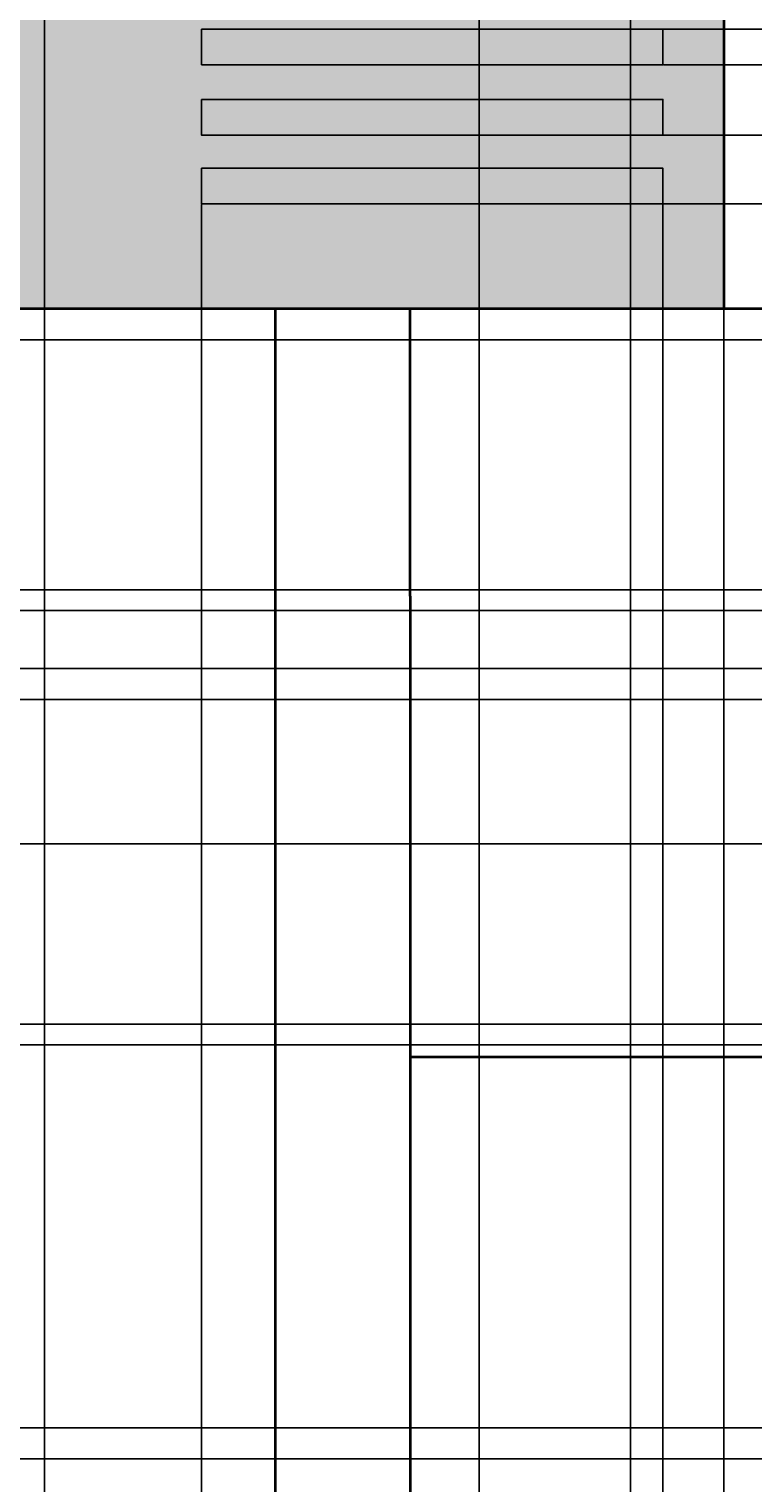
# Model space of a CAD drawing. Units: inches. Extents: x 62 to 566, y 66 to 528.
# Tile 13 of 20: x 373 to 443, y 158 to 298. Entities that reach past the tile are written whole.
import ezdxf

# ---------------------------------------------------------------- set-up
doc = ezdxf.new("R2010")
doc.units = ezdxf.units.IN
doc.header["$MEASUREMENT"] = 0
for name, color, linetype, lineweight in [('A-ANNO-DIMS', 2, 'Continuous', 18), ('A-DOOR', 4, 'Continuous', 25), ('A-ELEV', 7, 'Continuous', 35), ('A-GLAZ', 3, 'Continuous', 25), ('A-WALL-PATT', 8, 'Continuous', 13)]:
    doc.layers.add(name, color=color, linetype=linetype, lineweight=lineweight)
doc.styles.get("Standard").update_dxf_attribs({"font": 'arial.ttf'})
doc.dimstyles.get("Standard").update_dxf_attribs({"dimtxt": 0.75, "dimasz": 0.18, "dimexe": 0.18, "dimexo": 0.0625, "dimgap": 0.09, "dimtad": 0, "dimtih": 1, "dimtoh": 1, "dimdec": 4, "dimzin": 0, "dimdsep": 46, "dimlunit": 4, "dimtxsty": 'Standard', "dimcen": 0.09, "dimadec": 0, "dimazin": 0, "dimtfac": 1, "dimtdec": 4, "dimtofl": 0, "dimtmove": 0, "dimatfit": 3, "dimfxl": 1, "dimtolj": 1, "dimtzin": 0, "dimarcsym": 0})

# ---------------------------------------------------------------- blocks, each defined once
blk = doc.blocks.new('*D10')
at = {"layer": 'A-ANNO-DIMS', "color": 0, "lineweight": -2, "transparency": 16777216}
for p, q in [((396.43, 271.35), (396.43, 65.94)), ((316.21, 126.31), (316.21, 65.94)), ((316.39, 66.12), (354.97, 66.12)), ((396.25, 66.12), (357.67, 66.12))]:
    blk.add_line(p, q, dxfattribs=at)
at = {"layer": 'A-ANNO-DIMS', "color": 0, "transparency": 16777216}
for points in [[(316.39, 66.15), (316.39, 66.09), (316.21, 66.12)], [(396.25, 66.15), (396.25, 66.09), (396.43, 66.12)]]:
    blk.add_solid(points, dxfattribs=at)
at = {"layer": 'Defpoints', "color": 0, "transparency": 16777216}
for p in [(396.43, 271.41), (316.21, 126.37), (396.43, 66.12)]:
    blk.add_point(p, dxfattribs=at)
at = {"layer": 'A-ANNO-DIMS', "color": 0, "transparency": 16777216, "insert": (356.32, 66.12), "char_height": 0.75, "attachment_point": 5}
blk.add_mtext('\\A1;80.22', dxfattribs=at)
blk = doc.blocks.new('*D11')
at = {"layer": 'A-ANNO-DIMS', "color": 0, "lineweight": -2, "transparency": 16777216}
for p, q in [((396.43, 271.35), (396.43, 65.94)), ((409.43, 126.31), (409.43, 65.94)), ((396.61, 66.12), (402.34, 66.12)), ((409.25, 66.12), (403.52, 66.12))]:
    blk.add_line(p, q, dxfattribs=at)
at = {"layer": 'A-ANNO-DIMS', "color": 0, "transparency": 16777216}
for points in [[(396.61, 66.15), (396.61, 66.09), (396.43, 66.12)], [(409.25, 66.15), (409.25, 66.09), (409.43, 66.12)]]:
    blk.add_solid(points, dxfattribs=at)
at = {"layer": 'Defpoints', "color": 0, "transparency": 16777216}
for p in [(396.43, 271.41), (409.43, 126.37), (409.43, 66.12)]:
    blk.add_point(p, dxfattribs=at)
at = {"layer": 'A-ANNO-DIMS', "color": 0, "transparency": 16777216, "insert": (402.93, 66.12), "char_height": 0.75, "attachment_point": 5}
blk.add_mtext('\\A1;13', dxfattribs=at)
blk = doc.blocks.new('*D21')
at = {"layer": 'A-ANNO-DIMS', "color": 0, "lineweight": -2, "transparency": 16777216}
for p, q in [((374.2, 236.66), (564.47, 236.66)), ((564.29, 236.48), (564.29, 218.37)), ((564.29, 199.31), (564.29, 217.42)), ((474.18, 199.13), (564.47, 199.13))]:
    blk.add_line(p, q, dxfattribs=at)
at = {"layer": 'A-ANNO-DIMS', "color": 0, "transparency": 16777216}
for points in [[(564.26, 236.48), (564.32, 236.48), (564.29, 236.66)], [(564.26, 199.31), (564.32, 199.31), (564.29, 199.13)]]:
    blk.add_solid(points, dxfattribs=at)
at = {"layer": 'Defpoints', "color": 0, "transparency": 16777216}
for p in [(374.14, 236.66), (564.29, 236.66), (474.12, 199.13)]:
    blk.add_point(p, dxfattribs=at)
at = {"layer": 'A-ANNO-DIMS', "color": 0, "transparency": 16777216, "insert": (564.29, 217.9), "char_height": 0.75, "attachment_point": 5}
blk.add_mtext('\\A1;37.53', dxfattribs=at)
blk = doc.blocks.new('*D22')
at = {"layer": 'A-ANNO-DIMS', "color": 0, "lineweight": -2, "transparency": 16777216}
for p, q in [((540.1, 271.41), (564.47, 271.41)), ((564.29, 271.23), (564.29, 254.51)), ((564.29, 236.84), (564.29, 253.56)), ((374.2, 236.66), (564.47, 236.66))]:
    blk.add_line(p, q, dxfattribs=at)
at = {"layer": 'A-ANNO-DIMS', "color": 0, "transparency": 16777216}
for points in [[(564.26, 271.23), (564.32, 271.23), (564.29, 271.41)], [(564.26, 236.84), (564.32, 236.84), (564.29, 236.66)]]:
    blk.add_solid(points, dxfattribs=at)
at = {"layer": 'Defpoints', "color": 0, "transparency": 16777216}
for p in [(540.04, 271.41), (564.29, 271.41), (374.14, 236.66)]:
    blk.add_point(p, dxfattribs=at)
at = {"layer": 'A-ANNO-DIMS', "color": 0, "transparency": 16777216, "insert": (564.29, 254.04), "char_height": 0.75, "attachment_point": 5}
blk.add_mtext('\\A1;34.75', dxfattribs=at)
blk = doc.blocks.new('*D23')
at = {"layer": 'A-ANNO-DIMS', "color": 0, "lineweight": -2, "transparency": 16777216}
for p, q in [((374.2, 344.78), (564.47, 344.78)), ((564.29, 344.6), (564.29, 308.57)), ((564.29, 271.59), (564.29, 307.62)), ((540.1, 271.41), (564.47, 271.41))]:
    blk.add_line(p, q, dxfattribs=at)
at = {"layer": 'A-ANNO-DIMS', "color": 0, "transparency": 16777216}
for points in [[(564.26, 344.6), (564.32, 344.6), (564.29, 344.78)], [(564.26, 271.59), (564.32, 271.59), (564.29, 271.41)]]:
    blk.add_solid(points, dxfattribs=at)
at = {"layer": 'Defpoints', "color": 0, "transparency": 16777216}
for p in [(374.14, 344.78), (564.29, 344.78), (540.04, 271.41)]:
    blk.add_point(p, dxfattribs=at)
at = {"layer": 'A-ANNO-DIMS', "color": 0, "transparency": 16777216, "insert": (564.29, 308.1), "char_height": 0.75, "attachment_point": 5}
blk.add_mtext('\\A1;73.37', dxfattribs=at)
blk = doc.blocks.new('*D41')
at = {"layer": 'A-ANNO-DIMS', "color": 0, "lineweight": -2, "transparency": 16777216}
for p, q in [((316.21, 417.64), (316.21, 65.94)), ((374.14, 417.64), (374.14, 65.94)), ((316.39, 66.12), (343.82, 66.12)), ((373.96, 66.12), (346.53, 66.12))]:
    blk.add_line(p, q, dxfattribs=at)
at = {"layer": 'A-ANNO-DIMS', "color": 0, "transparency": 16777216}
for points in [[(316.39, 66.15), (316.39, 66.09), (316.21, 66.12)], [(373.96, 66.15), (373.96, 66.09), (374.14, 66.12)]]:
    blk.add_solid(points, dxfattribs=at)
at = {"layer": 'Defpoints', "color": 0, "transparency": 16777216}
for p in [(316.21, 417.71), (374.14, 417.71), (374.14, 66.12)]:
    blk.add_point(p, dxfattribs=at)
at = {"layer": 'A-ANNO-DIMS', "color": 0, "transparency": 16777216, "insert": (345.17, 66.12), "char_height": 0.75, "attachment_point": 5}
blk.add_mtext('\\A1;57.93', dxfattribs=at)
blk = doc.blocks.new('*D42')
at = {"layer": 'A-ANNO-DIMS', "color": 0, "lineweight": -2, "transparency": 16777216}
for p, q in [((416.08, 445.04), (416.08, 65.94)), ((374.14, 417.64), (374.14, 65.94)), ((374.32, 66.12), (393.74, 66.12)), ((415.9, 66.12), (396.48, 66.12))]:
    blk.add_line(p, q, dxfattribs=at)
at = {"layer": 'A-ANNO-DIMS', "color": 0, "transparency": 16777216}
for points in [[(374.32, 66.15), (374.32, 66.09), (374.14, 66.12)], [(415.9, 66.15), (415.9, 66.09), (416.08, 66.12)]]:
    blk.add_solid(points, dxfattribs=at)
at = {"layer": 'Defpoints', "color": 0, "transparency": 16777216}
for p in [(416.08, 445.11), (374.14, 417.71), (416.08, 66.12)]:
    blk.add_point(p, dxfattribs=at)
at = {"layer": 'A-ANNO-DIMS', "color": 0, "transparency": 16777216, "insert": (395.11, 66.12), "char_height": 0.75, "attachment_point": 5}
blk.add_mtext('\\A1;41.95', dxfattribs=at)
blk = doc.blocks.new('*D43')
at = {"layer": 'A-ANNO-DIMS', "color": 0, "lineweight": -2, "transparency": 16777216}
for p, q in [((416.08, 445.04), (416.08, 65.94)), ((430.69, 445.04), (430.69, 65.94)), ((416.26, 66.12), (422.14, 66.12)), ((430.51, 66.12), (424.64, 66.12))]:
    blk.add_line(p, q, dxfattribs=at)
at = {"layer": 'A-ANNO-DIMS', "color": 0, "transparency": 16777216}
for points in [[(416.26, 66.15), (416.26, 66.09), (416.08, 66.12)], [(430.51, 66.15), (430.51, 66.09), (430.69, 66.12)]]:
    blk.add_solid(points, dxfattribs=at)
at = {"layer": 'Defpoints', "color": 0, "transparency": 16777216}
for p in [(416.08, 445.11), (430.69, 445.11), (430.69, 66.12)]:
    blk.add_point(p, dxfattribs=at)
at = {"layer": 'A-ANNO-DIMS', "color": 0, "transparency": 16777216, "insert": (423.39, 66.12), "char_height": 0.75, "attachment_point": 5}
blk.add_mtext('\\A1;14.61', dxfattribs=at)
blk = doc.blocks.new('*D64')
at = {"layer": 'A-ANNO-DIMS', "color": 0, "lineweight": -2, "transparency": 16777216}
for p, q in [((371.14, 233.72), (371.14, 527.47)), ((371.32, 527.29), (372.3, 527.29)), ((373.96, 527.29), (372.97, 527.29)), ((374.14, 236.72), (374.14, 527.47))]:
    blk.add_line(p, q, dxfattribs=at)
at = {"layer": 'A-ANNO-DIMS', "color": 0, "transparency": 16777216}
for points in [[(371.32, 527.32), (371.32, 527.26), (371.14, 527.29)], [(373.96, 527.32), (373.96, 527.26), (374.14, 527.29)]]:
    blk.add_solid(points, dxfattribs=at)
at = {"layer": 'Defpoints', "color": 0, "transparency": 16777216}
for p in [(374.14, 527.29), (374.14, 236.66), (371.14, 233.66)]:
    blk.add_point(p, dxfattribs=at)
at = {"layer": 'A-ANNO-DIMS', "color": 0, "transparency": 16777216, "insert": (372.64, 527.29), "char_height": 0.75, "attachment_point": 5}
blk.add_mtext('\\A1;3', dxfattribs=at)
blk = doc.blocks.new('*D70')
at = {"layer": 'A-ANNO-DIMS', "color": 0, "lineweight": -2, "transparency": 16777216}
for p, q in [((329.73, 219.73), (564.47, 219.73)), ((564.29, 219.55), (564.29, 175.02)), ((564.29, 129.55), (564.29, 174.08)), ((371.2, 129.37), (564.47, 129.37))]:
    blk.add_line(p, q, dxfattribs=at)
at = {"layer": 'A-ANNO-DIMS', "color": 0, "transparency": 16777216}
for points in [[(564.26, 219.55), (564.32, 219.55), (564.29, 219.73)], [(564.26, 129.55), (564.32, 129.55), (564.29, 129.37)]]:
    blk.add_solid(points, dxfattribs=at)
at = {"layer": 'Defpoints', "color": 0, "transparency": 16777216}
for p in [(329.67, 219.73), (564.29, 219.73), (371.14, 129.37)]:
    blk.add_point(p, dxfattribs=at)
at = {"layer": 'A-ANNO-DIMS', "color": 0, "transparency": 16777216, "insert": (564.29, 174.55), "char_height": 0.75, "attachment_point": 5}
blk.add_mtext('\\A1;90.36', dxfattribs=at)
blk = doc.blocks.new('*D71')
at = {"layer": 'A-ANNO-DIMS', "color": 0, "lineweight": -2, "transparency": 16777216}
for p, q in [((371.2, 233.66), (564.47, 233.66)), ((564.29, 233.48), (564.29, 227.17)), ((564.29, 219.91), (564.29, 226.22)), ((329.73, 219.73), (564.47, 219.73))]:
    blk.add_line(p, q, dxfattribs=at)
at = {"layer": 'A-ANNO-DIMS', "color": 0, "transparency": 16777216}
for points in [[(564.26, 233.48), (564.32, 233.48), (564.29, 233.66)], [(564.26, 219.91), (564.32, 219.91), (564.29, 219.73)]]:
    blk.add_solid(points, dxfattribs=at)
at = {"layer": 'Defpoints', "color": 0, "transparency": 16777216}
for p in [(371.14, 233.66), (564.29, 233.66), (329.67, 219.73)]:
    blk.add_point(p, dxfattribs=at)
at = {"layer": 'A-ANNO-DIMS', "color": 0, "transparency": 16777216, "insert": (564.29, 226.7), "char_height": 0.75, "attachment_point": 5}
blk.add_mtext('\\A1;13.93', dxfattribs=at)
blk = doc.blocks.new('*D72')
at = {"layer": 'A-ANNO-DIMS', "color": 0, "lineweight": -2, "transparency": 16777216}
for p, q in [((374.2, 236.66), (564.47, 236.66)), ((564.29, 236.48), (564.29, 235.63)), ((564.29, 233.84), (564.29, 234.69)), ((371.2, 233.66), (564.47, 233.66))]:
    blk.add_line(p, q, dxfattribs=at)
at = {"layer": 'A-ANNO-DIMS', "color": 0, "transparency": 16777216}
for points in [[(564.26, 236.48), (564.32, 236.48), (564.29, 236.66)], [(564.26, 233.84), (564.32, 233.84), (564.29, 233.66)]]:
    blk.add_solid(points, dxfattribs=at)
at = {"layer": 'Defpoints', "color": 0, "transparency": 16777216}
for p in [(374.14, 236.66), (564.29, 236.66), (371.14, 233.66)]:
    blk.add_point(p, dxfattribs=at)
at = {"layer": 'A-ANNO-DIMS', "color": 0, "transparency": 16777216, "insert": (564.29, 235.16), "char_height": 0.75, "attachment_point": 5}
blk.add_mtext('\\A1;3', dxfattribs=at)
blk = doc.blocks.new('*D85')
at = {"layer": 'A-ANNO-DIMS', "color": 0, "lineweight": -2, "transparency": 16777216}
for p, q in [((389.29, 281.45), (389.29, 65.94)), ((341.26, 279.98), (341.26, 65.94)), ((341.44, 66.12), (363.91, 66.12)), ((389.11, 66.12), (366.64, 66.12))]:
    blk.add_line(p, q, dxfattribs=at)
at = {"layer": 'A-ANNO-DIMS', "color": 0, "transparency": 16777216}
for points in [[(341.44, 66.15), (341.44, 66.09), (341.26, 66.12)], [(389.11, 66.15), (389.11, 66.09), (389.29, 66.12)]]:
    blk.add_solid(points, dxfattribs=at)
at = {"layer": 'Defpoints', "color": 0, "transparency": 16777216}
for p in [(389.29, 281.51), (341.26, 280.04), (389.29, 66.12)]:
    blk.add_point(p, dxfattribs=at)
at = {"layer": 'A-ANNO-DIMS', "color": 0, "transparency": 16777216, "insert": (365.27, 66.12), "char_height": 0.75, "attachment_point": 5}
blk.add_mtext('\\A1;48.02', dxfattribs=at)
blk = doc.blocks.new('*D86')
at = {"layer": 'A-ANNO-DIMS', "color": 0, "lineweight": -2, "transparency": 16777216}
for p, q in [((389.29, 281.45), (389.29, 65.94)), ((433.81, 281.45), (433.81, 65.94)), ((389.47, 66.12), (409.89, 66.12)), ((433.63, 66.12), (413.21, 66.12))]:
    blk.add_line(p, q, dxfattribs=at)
at = {"layer": 'A-ANNO-DIMS', "color": 0, "transparency": 16777216}
for points in [[(389.47, 66.15), (389.47, 66.09), (389.29, 66.12)], [(433.63, 66.15), (433.63, 66.09), (433.81, 66.12)]]:
    blk.add_solid(points, dxfattribs=at)
at = {"layer": 'Defpoints', "color": 0, "transparency": 16777216}
for p in [(389.29, 281.51), (433.81, 281.51), (433.81, 66.12)]:
    blk.add_point(p, dxfattribs=at)
at = {"layer": 'A-ANNO-DIMS', "color": 0, "transparency": 16777216, "insert": (411.55, 66.12), "char_height": 0.75, "attachment_point": 5}
blk.add_mtext('\\A1;44.524', dxfattribs=at)
blk = doc.blocks.new('*D87')
at = {"layer": 'A-ANNO-DIMS', "color": 0, "lineweight": -2, "transparency": 16777216}
for p, q in [((433.81, 281.45), (433.81, 65.94)), ((439.69, 271.35), (439.69, 65.94)), ((433.99, 66.12), (435.39, 66.12)), ((439.51, 66.12), (438.11, 66.12))]:
    blk.add_line(p, q, dxfattribs=at)
at = {"layer": 'A-ANNO-DIMS', "color": 0, "transparency": 16777216}
for points in [[(433.99, 66.15), (433.99, 66.09), (433.81, 66.12)], [(439.51, 66.15), (439.51, 66.09), (439.69, 66.12)]]:
    blk.add_solid(points, dxfattribs=at)
at = {"layer": 'Defpoints', "color": 0, "transparency": 16777216}
for p in [(433.81, 281.51), (439.69, 271.41), (439.69, 66.12)]:
    blk.add_point(p, dxfattribs=at)
at = {"layer": 'A-ANNO-DIMS', "color": 0, "transparency": 16777216, "insert": (436.75, 66.12), "char_height": 0.75, "attachment_point": 5}
blk.add_mtext('\\A1;5.878', dxfattribs=at)
blk = doc.blocks.new('*D88')
at = {"layer": 'A-ANNO-DIMS', "color": 0, "lineweight": -2, "transparency": 16777216}
for p, q in [((433.87, 281.51), (564.47, 281.51)), ((564.29, 281.33), (564.29, 276.94)), ((564.29, 271.59), (564.29, 275.99)), ((439.75, 271.41), (564.47, 271.41))]:
    blk.add_line(p, q, dxfattribs=at)
at = {"layer": 'A-ANNO-DIMS', "color": 0, "transparency": 16777216}
for points in [[(564.26, 281.33), (564.32, 281.33), (564.29, 281.51)], [(564.26, 271.59), (564.32, 271.59), (564.29, 271.41)]]:
    blk.add_solid(points, dxfattribs=at)
at = {"layer": 'Defpoints', "color": 0, "transparency": 16777216}
for p in [(433.81, 281.51), (564.29, 281.51), (439.69, 271.41)]:
    blk.add_point(p, dxfattribs=at)
at = {"layer": 'A-ANNO-DIMS', "color": 0, "transparency": 16777216, "insert": (564.29, 276.46), "char_height": 0.75, "attachment_point": 5}
blk.add_mtext('\\A1;10.1', dxfattribs=at)
blk = doc.blocks.new('*D89')
at = {"layer": 'A-ANNO-DIMS', "color": 0, "lineweight": -2, "transparency": 16777216}
for p, q in [((433.87, 288.16), (564.47, 288.16)), ((564.29, 287.98), (564.29, 285.31)), ((564.29, 281.69), (564.29, 284.36)), ((433.87, 281.51), (564.47, 281.51))]:
    blk.add_line(p, q, dxfattribs=at)
at = {"layer": 'A-ANNO-DIMS', "color": 0, "transparency": 16777216}
for points in [[(564.26, 287.98), (564.32, 287.98), (564.29, 288.16)], [(564.26, 281.69), (564.32, 281.69), (564.29, 281.51)]]:
    blk.add_solid(points, dxfattribs=at)
at = {"layer": 'Defpoints', "color": 0, "transparency": 16777216}
for p in [(433.81, 288.16), (564.29, 288.16), (433.81, 281.51)]:
    blk.add_point(p, dxfattribs=at)
at = {"layer": 'A-ANNO-DIMS', "color": 0, "transparency": 16777216, "insert": (564.29, 284.83), "char_height": 0.75, "attachment_point": 5}
blk.add_mtext('\\A1;6.643', dxfattribs=at)
blk = doc.blocks.new('*D90')
at = {"layer": 'A-ANNO-DIMS', "color": 0, "lineweight": -2, "transparency": 16777216}
for p, q in [((433.87, 294.95), (564.47, 294.95)), ((564.29, 294.77), (564.29, 292.03)), ((564.29, 288.34), (564.29, 291.08)), ((433.87, 288.16), (564.47, 288.16))]:
    blk.add_line(p, q, dxfattribs=at)
at = {"layer": 'A-ANNO-DIMS', "color": 0, "transparency": 16777216}
for points in [[(564.26, 294.77), (564.32, 294.77), (564.29, 294.95)], [(564.26, 288.34), (564.32, 288.34), (564.29, 288.16)]]:
    blk.add_solid(points, dxfattribs=at)
at = {"layer": 'Defpoints', "color": 0, "transparency": 16777216}
for p in [(433.81, 294.95), (564.29, 294.95), (433.81, 288.16)]:
    blk.add_point(p, dxfattribs=at)
at = {"layer": 'A-ANNO-DIMS', "color": 0, "transparency": 16777216, "insert": (564.29, 291.55), "char_height": 0.75, "attachment_point": 5}
blk.add_mtext('\\A1;6.795', dxfattribs=at)
blk = doc.blocks.new('*D91')
at = {"layer": 'A-ANNO-DIMS', "color": 0, "lineweight": -2, "transparency": 16777216}
for p, q in [((433.87, 298.4), (564.47, 298.4)), ((564.29, 298.22), (564.29, 297.15)), ((564.29, 295.13), (564.29, 296.2)), ((433.87, 294.95), (564.47, 294.95))]:
    blk.add_line(p, q, dxfattribs=at)
at = {"layer": 'A-ANNO-DIMS', "color": 0, "transparency": 16777216}
for points in [[(564.26, 298.22), (564.32, 298.22), (564.29, 298.4)], [(564.26, 295.13), (564.32, 295.13), (564.29, 294.95)]]:
    blk.add_solid(points, dxfattribs=at)
at = {"layer": 'Defpoints', "color": 0, "transparency": 16777216}
for p in [(433.81, 298.4), (564.29, 298.4), (433.81, 294.95)]:
    blk.add_point(p, dxfattribs=at)
at = {"layer": 'A-ANNO-DIMS', "color": 0, "transparency": 16777216, "insert": (564.29, 296.67), "char_height": 0.75, "attachment_point": 5}
blk.add_mtext('\\A1;3.449', dxfattribs=at)
blk = doc.blocks.new('*D121')
at = {"layer": 'A-ANNO-DIMS', "color": 0, "lineweight": -2, "transparency": 16777216}
for p, q in [((272.12, 160.35), (564.47, 160.35)), ((564.29, 160.17), (564.29, 158.34)), ((564.29, 155.56), (564.29, 157.39)), ((267.86, 155.38), (564.47, 155.38))]:
    blk.add_line(p, q, dxfattribs=at)
at = {"layer": 'A-ANNO-DIMS', "color": 0, "transparency": 16777216}
for points in [[(564.26, 160.17), (564.32, 160.17), (564.29, 160.35)], [(564.26, 155.56), (564.32, 155.56), (564.29, 155.38)]]:
    blk.add_solid(points, dxfattribs=at)
at = {"layer": 'Defpoints', "color": 0, "transparency": 16777216}
for p in [(272.06, 160.35), (564.29, 160.35), (267.79, 155.38)]:
    blk.add_point(p, dxfattribs=at)
at = {"layer": 'A-ANNO-DIMS', "color": 0, "transparency": 16777216, "insert": (564.29, 157.87), "char_height": 0.75, "attachment_point": 5}
blk.add_mtext('\\A1;4.975', dxfattribs=at)
blk = doc.blocks.new('*D122')
at = {"layer": 'A-ANNO-DIMS', "color": 0, "lineweight": -2, "transparency": 16777216}
for p, q in [((269.12, 163.35), (564.47, 163.35)), ((564.29, 163.17), (564.29, 162.33)), ((272.12, 160.35), (564.47, 160.35)), ((564.29, 160.53), (564.29, 161.38))]:
    blk.add_line(p, q, dxfattribs=at)
at = {"layer": 'A-ANNO-DIMS', "color": 0, "transparency": 16777216}
for points in [[(564.26, 163.17), (564.32, 163.17), (564.29, 163.35)], [(564.26, 160.53), (564.32, 160.53), (564.29, 160.35)]]:
    blk.add_solid(points, dxfattribs=at)
at = {"layer": 'Defpoints', "color": 0, "transparency": 16777216}
for p in [(269.06, 163.35), (564.29, 163.35), (272.06, 160.35)]:
    blk.add_point(p, dxfattribs=at)
at = {"layer": 'A-ANNO-DIMS', "color": 0, "transparency": 16777216, "insert": (564.29, 161.85), "char_height": 0.75, "attachment_point": 5}
blk.add_mtext('\\A1;3', dxfattribs=at)
blk = doc.blocks.new('*D123')
at = {"layer": 'A-ANNO-DIMS', "color": 0, "lineweight": -2, "transparency": 16777216}
for p, q in [((269.12, 200.32), (564.47, 200.32)), ((564.29, 200.14), (564.29, 182.31)), ((564.29, 163.53), (564.29, 181.37)), ((269.12, 163.35), (564.47, 163.35))]:
    blk.add_line(p, q, dxfattribs=at)
at = {"layer": 'A-ANNO-DIMS', "color": 0, "transparency": 16777216}
for points in [[(564.26, 200.14), (564.32, 200.14), (564.29, 200.32)], [(564.26, 163.53), (564.32, 163.53), (564.29, 163.35)]]:
    blk.add_solid(points, dxfattribs=at)
at = {"layer": 'Defpoints', "color": 0, "transparency": 16777216}
for p in [(269.06, 200.32), (564.29, 200.32), (269.06, 163.35)]:
    blk.add_point(p, dxfattribs=at)
at = {"layer": 'A-ANNO-DIMS', "color": 0, "transparency": 16777216, "insert": (564.29, 181.84), "char_height": 0.75, "attachment_point": 5}
blk.add_mtext('\\A1;36.97', dxfattribs=at)
blk = doc.blocks.new('*D124')
at = {"layer": 'A-ANNO-DIMS', "color": 0, "lineweight": -2, "transparency": 16777216}
for p, q in [((269.12, 202.32), (564.47, 202.32)), ((564.29, 202.14), (564.29, 201.79)), ((564.29, 200.5), (564.29, 200.86)), ((269.12, 200.32), (564.47, 200.32))]:
    blk.add_line(p, q, dxfattribs=at)
at = {"layer": 'A-ANNO-DIMS', "color": 0, "transparency": 16777216}
for points in [[(564.26, 202.14), (564.32, 202.14), (564.29, 202.32)], [(564.26, 200.5), (564.32, 200.5), (564.29, 200.32)]]:
    blk.add_solid(points, dxfattribs=at)
at = {"layer": 'Defpoints', "color": 0, "transparency": 16777216}
for p in [(269.06, 202.32), (564.29, 202.32), (269.06, 200.32)]:
    blk.add_point(p, dxfattribs=at)
at = {"layer": 'A-ANNO-DIMS', "color": 0, "transparency": 16777216, "insert": (564.29, 201.32), "char_height": 0.75, "attachment_point": 5}
blk.add_mtext('\\A1;2', dxfattribs=at)
blk = doc.blocks.new('*D125')
at = {"layer": 'A-ANNO-DIMS', "color": 0, "lineweight": -2, "transparency": 16777216}
for p, q in [((269.12, 242.25), (564.47, 242.25)), ((564.29, 242.07), (564.29, 222.76)), ((564.29, 202.5), (564.29, 221.81)), ((269.12, 202.32), (564.47, 202.32))]:
    blk.add_line(p, q, dxfattribs=at)
at = {"layer": 'A-ANNO-DIMS', "color": 0, "transparency": 16777216}
for points in [[(564.26, 242.07), (564.32, 242.07), (564.29, 242.25)], [(564.26, 202.5), (564.32, 202.5), (564.29, 202.32)]]:
    blk.add_solid(points, dxfattribs=at)
at = {"layer": 'Defpoints', "color": 0, "transparency": 16777216}
for p in [(269.06, 242.25), (564.29, 242.25), (269.06, 202.32)]:
    blk.add_point(p, dxfattribs=at)
at = {"layer": 'A-ANNO-DIMS', "color": 0, "transparency": 16777216, "insert": (564.29, 222.29), "char_height": 0.75, "attachment_point": 5}
blk.add_mtext('\\A1;39.93', dxfattribs=at)
blk = doc.blocks.new('*D126')
at = {"layer": 'A-ANNO-DIMS', "color": 0, "lineweight": -2, "transparency": 16777216}
for p, q in [((269.12, 244.25), (564.47, 244.25)), ((564.29, 244.07), (564.29, 243.72)), ((269.12, 242.25), (564.47, 242.25)), ((564.29, 242.43), (564.29, 242.78))]:
    blk.add_line(p, q, dxfattribs=at)
at = {"layer": 'A-ANNO-DIMS', "color": 0, "transparency": 16777216}
for points in [[(564.26, 244.07), (564.32, 244.07), (564.29, 244.25)], [(564.26, 242.43), (564.32, 242.43), (564.29, 242.25)]]:
    blk.add_solid(points, dxfattribs=at)
at = {"layer": 'Defpoints', "color": 0, "transparency": 16777216}
for p in [(269.06, 244.25), (564.29, 244.25), (269.06, 242.25)]:
    blk.add_point(p, dxfattribs=at)
at = {"layer": 'A-ANNO-DIMS', "color": 0, "transparency": 16777216, "insert": (564.29, 243.25), "char_height": 0.75, "attachment_point": 5}
blk.add_mtext('\\A1;2', dxfattribs=at)
blk = doc.blocks.new('*D127')
at = {"layer": 'A-ANNO-DIMS', "color": 0, "lineweight": -2, "transparency": 16777216}
for p, q in [((269.12, 268.41), (564.47, 268.41)), ((564.29, 268.23), (564.29, 256.8)), ((564.29, 244.43), (564.29, 255.86)), ((269.12, 244.25), (564.47, 244.25))]:
    blk.add_line(p, q, dxfattribs=at)
at = {"layer": 'A-ANNO-DIMS', "color": 0, "transparency": 16777216}
for points in [[(564.26, 268.23), (564.32, 268.23), (564.29, 268.41)], [(564.26, 244.43), (564.32, 244.43), (564.29, 244.25)]]:
    blk.add_solid(points, dxfattribs=at)
at = {"layer": 'Defpoints', "color": 0, "transparency": 16777216}
for p in [(269.06, 268.41), (564.29, 268.41), (269.06, 244.25)]:
    blk.add_point(p, dxfattribs=at)
at = {"layer": 'A-ANNO-DIMS', "color": 0, "transparency": 16777216, "insert": (564.29, 256.33), "char_height": 0.75, "attachment_point": 5}
blk.add_mtext('\\A1;24.16', dxfattribs=at)
blk = doc.blocks.new('*D128')
at = {"layer": 'A-ANNO-DIMS', "color": 0, "lineweight": -2, "transparency": 16777216}
for p, q in [((272.12, 271.41), (564.47, 271.41)), ((564.29, 271.23), (564.29, 270.39)), ((269.12, 268.41), (564.47, 268.41)), ((564.29, 268.59), (564.29, 269.44))]:
    blk.add_line(p, q, dxfattribs=at)
at = {"layer": 'A-ANNO-DIMS', "color": 0, "transparency": 16777216}
for points in [[(564.26, 271.23), (564.32, 271.23), (564.29, 271.41)], [(564.26, 268.59), (564.32, 268.59), (564.29, 268.41)]]:
    blk.add_solid(points, dxfattribs=at)
at = {"layer": 'Defpoints', "color": 0, "transparency": 16777216}
for p in [(272.06, 271.41), (564.29, 271.41), (269.06, 268.41)]:
    blk.add_point(p, dxfattribs=at)
at = {"layer": 'A-ANNO-DIMS', "color": 0, "transparency": 16777216, "insert": (564.29, 269.91), "char_height": 0.75, "attachment_point": 5}
blk.add_mtext('\\A1;3', dxfattribs=at)

msp = doc.modelspace()

# ---------------------------------------------------------------- hatches: boundary and pattern name
at = {"layer": 'A-WALL-PATT'}
h = msp.add_hatch(color=256, dxfattribs=at)
h.dxf.hatch_style = 1
h.paths.add_polyline_path([(416.0836, 462.0423), (125.9418, 462.0423), (125.9418, 414.3686), (125.9418, 270.3686), (125.9418, 126.3686), (142.3851, 126.3686), (142.3851, 270.3686), (142.3851, 414.3686), (142.3851, 445.1064), (284.2021, 445.1064), (416.0836, 445.1064)])
h.paths.add_polyline_path([(435.3945, 503.0423), (426.3652, 503.0423), (120.4058, 503.0423), (120.4058, 501.0423), (125.9418, 501.0423), (416.0836, 501.0423), (426.3652, 501.0423), (430.6938, 501.0423), (435.3945, 501.0423)])
h.paths.add_polyline_path([(439.6878, 352.4848), (392.4793, 352.4848), (392.4793, 307.4128), (217.2752, 307.4128), (217.2752, 295.4098), (217.2752, 271.4128), (272.0586, 271.4128), (439.6878, 271.4128)])
h.paths.add_polyline_path([(248.0143, 297.1682), (255.6783, 297.1682), (255.6783, 280.0423), (248.0143, 280.0423)], flags=16)
h.paths.add_polyline_path([(235.4641, 280.0423), (227.8001, 280.0423), (227.8001, 297.1682), (235.4641, 297.1682)], flags=16)
h.paths.add_polyline_path([(270.4427, 297.1682), (278.1067, 297.1682), (278.1067, 280.0423), (270.4427, 280.0423)], flags=16)
h.paths.add_polyline_path([(296.3755, 297.1682), (304.0395, 297.1682), (304.0395, 280.0423), (296.3755, 280.0423)], flags=16)
h.paths.add_polyline_path([(319.2543, 297.1682), (326.9183, 297.1682), (326.9183, 280.0423), (319.2543, 280.0423)], flags=16)
h.paths.add_polyline_path([(341.2622, 297.1682), (348.9262, 297.1682), (348.9262, 280.0423), (341.2622, 280.0423)], flags=16)
h.paths.add_polyline_path([(389.2857, 298.3985), (433.8102, 298.3985), (433.8102, 294.9497), (389.2857, 294.9497)], flags=16)
h.paths.add_polyline_path([(389.2857, 291.6038), (433.8102, 291.6038), (433.8102, 288.155), (389.2857, 288.155)], flags=16)
h.paths.add_polyline_path([(389.2857, 284.9607), (433.8102, 284.9607), (433.8102, 281.5119), (389.2857, 281.5119)], flags=16)
h.paths.add_polyline_path([(403.5849, 311.4736), (403.5849, 317.4388), (433.1636, 317.4388), (433.1636, 311.4736)], flags=16)
h.paths.add_polyline_path([(403.5849, 323.1329), (403.5849, 329.0982), (433.1636, 329.0982), (433.1636, 323.1329)], flags=16)
h.paths.add_polyline_path([(403.5849, 334.5211), (403.5849, 340.4863), (433.1636, 340.4863), (433.1636, 334.5211)], flags=16)
h.paths.add_polyline_path([(272.0586, 160.3545), (217.2752, 160.3545), (217.2752, 129.0504), (217.2752, 126.3686), (272.0586, 126.3686)], flags=17)
h.paths.add_polyline_path([(220.5897, 149.5749), (220.5897, 152.296), (267.7931, 152.296), (267.7931, 149.5749)], flags=16)
h.paths.add_polyline_path([(267.7931, 146.6724), (267.7931, 143.9513), (220.5897, 143.9513), (220.5897, 146.6724)], flags=16)
h.paths.add_polyline_path([(220.5897, 155.3799), (220.5897, 158.101), (267.7931, 158.101), (267.7931, 155.3799)], flags=16)
h.paths.add_polyline_path([(267.7931, 140.686), (267.7931, 137.9649), (220.5897, 137.9649), (220.5897, 140.686)], flags=16)
h.paths.add_polyline_path([(267.7931, 135.516), (267.7931, 132.7949), (220.5897, 132.7949), (220.5897, 135.516)], flags=16)
h = msp.add_hatch(color=256, dxfattribs=at)
h.dxf.hatch_style = 1
h.paths.add_polyline_path([(416.0836, 501.0423), (282.3509, 501.0423), (282.3509, 465.0423), (416.0836, 465.0423)])
h.paths.add_polyline_path([(284.2021, 420.597), (272.0586, 420.597), (272.0586, 309.5388), (272.0586, 307.4128), (284.2021, 307.4128)], flags=17)
h.paths.add_polyline_path([(284.2021, 445.1064), (142.3851, 445.1064), (142.3851, 414.3686), (142.3851, 270.3686), (142.3851, 126.3686), (163.6548, 126.3686), (163.6548, 270.5016), (163.6548, 414.5016), (163.6548, 427.4752), (284.2021, 427.4752)])
h.paths.add_polyline_path([(235.4641, 297.1682), (227.8001, 297.1682), (227.8001, 280.0423), (235.4641, 280.0423)], flags=17)
h.paths.add_polyline_path([(255.6783, 297.1682), (248.0143, 297.1682), (248.0143, 280.0423), (255.6783, 280.0423)], flags=17)
h.paths.add_polyline_path([(278.1067, 297.1682), (270.4427, 297.1682), (270.4427, 280.0423), (278.1067, 280.0423)], flags=17)
h.paths.add_polyline_path([(304.0395, 297.1682), (296.3755, 297.1682), (296.3755, 280.0423), (304.0395, 280.0423)])
h.paths.add_polyline_path([(326.9183, 297.1682), (319.2543, 297.1682), (319.2543, 280.0423), (326.9183, 280.0423)])
h.paths.add_polyline_path([(348.9262, 297.1682), (341.2622, 297.1682), (341.2622, 280.0423), (348.9262, 280.0423)])
h.paths.add_polyline_path([(433.8102, 284.9607), (389.2857, 284.9607), (389.2857, 281.5119), (433.8102, 281.5119)])
h.paths.add_polyline_path([(433.8102, 291.6038), (389.2857, 291.6038), (389.2857, 288.155), (433.8102, 288.155)])
h.paths.add_polyline_path([(433.8102, 298.3985), (389.2857, 298.3985), (389.2857, 294.9497), (433.8102, 294.9497)])
h.paths.add_polyline_path([(433.1636, 317.4388), (403.5849, 317.4388), (403.5849, 311.4736), (433.1636, 311.4736)])
h.paths.add_polyline_path([(433.1636, 329.0982), (403.5849, 329.0982), (403.5849, 323.1329), (433.1636, 323.1329)])
h.paths.add_polyline_path([(433.1636, 340.4863), (403.5849, 340.4863), (403.5849, 334.5211), (433.1636, 334.5211)])
h.paths.add_polyline_path([(284.2021, 271.4128), (272.0586, 271.4128), (272.0586, 160.3545), (272.0586, 126.3686), (284.2021, 126.3686)])
h.paths.add_polyline_path([(267.7931, 158.101), (220.5897, 158.101), (220.5897, 155.3799), (267.7931, 155.3799)], flags=17)
h.paths.add_polyline_path([(267.7931, 152.296), (220.5897, 152.296), (220.5897, 149.5749), (267.7931, 149.5749)], flags=17)
h.paths.add_polyline_path([(267.7931, 146.6724), (220.5897, 146.6724), (220.5897, 143.9513), (267.7931, 143.9513)], flags=17)
h.paths.add_polyline_path([(267.7931, 140.686), (220.5897, 140.686), (220.5897, 137.9649), (267.7931, 137.9649)], flags=17)
h.paths.add_polyline_path([(267.7931, 135.516), (220.5897, 135.516), (220.5897, 132.7949), (267.7931, 132.7949)], flags=17)
h.paths.add_polyline_path([(148.2354, 493.4274), (140.5713, 493.4274), (140.5713, 476.3015), (148.2354, 476.3015)])
h.paths.add_polyline_path([(163.2545, 493.4274), (155.5905, 493.4274), (155.5905, 476.3015), (163.2545, 476.3015)])
h.paths.add_polyline_path([(177.9243, 493.7764), (170.2603, 493.7764), (170.2603, 476.6506), (177.9243, 476.6506)])
h.paths.add_polyline_path([(193.9913, 493.7764), (186.3273, 493.7764), (186.3273, 476.6506), (193.9913, 476.6506)])
h.paths.add_polyline_path([(209.709, 493.7764), (202.045, 493.7764), (202.045, 476.6506), (209.709, 476.6506)])

# ---------------------------------------------------------------- linework, layer by layer
at = {"layer": 'A-DOOR'}
msp.add_lwpolyline([(316.2101, 236.6618), (374.1373, 236.6618), (374.1373, 126.3686), (316.2101, 126.3686)], close=True, dxfattribs=at)
at = {"layer": 'A-ELEV'}
for p, q in [((439.6878, 352.4848), (439.6878, 271.4128)), ((217.2752, 271.4128), (540.0368, 271.4128)), ((396.433, 126.3686), (396.433, 271.4128)), ((409.433, 243.6488), (409.433, 271.4128)), ((409.433, 243.6488), (409.433, 126.3686)), ((474.1214, 199.1332), (409.433, 199.1332))]:
    msp.add_line(p, q, dxfattribs=at)
at = {"layer": 'A-GLAZ'}
for points in [[(389.2857, 298.3985), (433.8102, 298.3985), (433.8102, 294.9497), (389.2857, 294.9497)], [(389.2857, 291.6038), (433.8102, 291.6038), (433.8102, 288.155), (389.2857, 288.155)], [(389.2857, 284.9607), (433.8102, 284.9607), (433.8102, 281.5119), (389.2857, 281.5119)]]:
    msp.add_lwpolyline(points, close=True, dxfattribs=at)

# ---------------------------------------------------------------- dimensions: what is measured, and where the dimension line sits
at = {"layer": 'A-ANNO-DIMS'}
for base, p1, p2, override, picture, middle in [((374.1373, 527.2923), (371.1373, 233.6618), (374.1373, 236.6618), {"dimdec": 0, "dimlfac": 1, "dimrnd": 0, "dimzin": 0, "dimdsep": 46, "dimlunit": 2}, '*D64', (372.6373, 527.2923)), ((416.0836, 66.1186), (374.1373, 417.7059), (416.0836, 445.1064), {"dimdec": 2, "dimlfac": 1, "dimrnd": 0, "dimzin": 0, "dimdsep": 46, "dimlunit": 2}, '*D42', (395.1104, 66.1186)), ((430.6938, 66.1186), (416.0836, 445.1064), (430.6938, 445.1064), {"dimdec": 2, "dimlfac": 1, "dimrnd": 0, "dimzin": 0, "dimdsep": 46, "dimlunit": 2}, '*D43', (423.3887, 66.1186)), ((374.1373, 66.1186), (316.2101, 417.7059), (374.1373, 417.7059), {"dimdec": 2, "dimlfac": 1, "dimrnd": 0, "dimzin": 0, "dimdsep": 46, "dimlunit": 2}, '*D41', (345.1737, 66.1186)), ((389.2857, 66.1186), (341.2622, 280.0423), (389.2857, 281.5119), {"dimdec": 2, "dimlfac": 1, "dimrnd": 0, "dimzin": 0, "dimdsep": 46, "dimlunit": 2}, '*D85', (365.2739, 66.1186)), ((433.81015, 66.11861), (389.28567, 281.51192), (433.81015, 281.51192), {"dimdec": 3, "dimlfac": 1, "dimrnd": 0, "dimzin": 0, "dimdsep": 46, "dimlunit": 2}, '*D86', (411.54791, 66.11861)), ((439.6878, 66.1186), (433.8102, 281.5119), (439.6878, 271.4128), {"dimdec": 3, "dimlfac": 1, "dimrnd": 0, "dimzin": 0, "dimdsep": 46, "dimlunit": 2}, '*D87', (436.749, 66.1186)), ((396.433, 66.1186), (316.2101, 126.3686), (396.433, 271.4128), {"dimdec": 2, "dimlfac": 1, "dimrnd": 0, "dimzin": 0, "dimdsep": 46, "dimlunit": 2}, '*D10', (356.3216, 66.1186)), ((409.433, 66.1186), (396.433, 271.4128), (409.433, 126.3686), {"dimdec": 0, "dimlfac": 1, "dimrnd": 0, "dimzin": 0, "dimdsep": 46, "dimlunit": 2}, '*D11', (402.933, 66.1186))]:
    dim = msp.add_linear_dim(base=base, p1=p1, p2=p2, dimstyle='Standard', override=override, dxfattribs=at)
    dim.commit()
    dim.dimension.update_dxf_attribs({"geometry": picture, "text_midpoint": middle})
for base, p1, p2, override, picture, middle in [((564.2868, 344.7821), (540.0368, 271.4128), (374.1373, 344.7821), {"dimdec": 2, "dimlfac": 1, "dimrnd": 0, "dimzin": 0, "dimdsep": 46, "dimlunit": 2}, '*D23', (564.2868, 308.0974)), ((564.2868, 298.3985), (433.8102, 294.9497), (433.8102, 298.3985), {"dimdec": 3, "dimlfac": 1, "dimrnd": 0, "dimzin": 0, "dimdsep": 46, "dimlunit": 2}, '*D91', (564.2868, 296.6741)), ((564.2868, 294.9497), (433.8102, 288.155), (433.8102, 294.9497), {"dimdec": 3, "dimlfac": 1, "dimrnd": 0, "dimzin": 0, "dimdsep": 46, "dimlunit": 2}, '*D90', (564.2868, 291.5524)), ((564.2868, 288.155), (433.8102, 281.5119), (433.8102, 288.155), {"dimdec": 3, "dimlfac": 1, "dimrnd": 0, "dimzin": 0, "dimdsep": 46, "dimlunit": 2}, '*D89', (564.2868, 284.8335)), ((564.2868, 281.5119), (439.6878, 271.4128), (433.8102, 281.5119), {"dimdec": 1, "dimlfac": 1, "dimrnd": 0, "dimzin": 0, "dimdsep": 46, "dimlunit": 2}, '*D88', (564.2868, 276.4623)), ((564.2868, 271.4128), (269.0586, 268.4128), (272.0586, 271.4128), {"dimdec": 0, "dimlfac": 1, "dimrnd": 0, "dimzin": 0, "dimdsep": 46, "dimlunit": 2}, '*D128', (564.2868, 269.9128)), ((564.2868, 271.4128), (374.1373, 236.6618), (540.0368, 271.4128), {"dimdec": 2, "dimlfac": 1, "dimrnd": 0, "dimzin": 0, "dimdsep": 46, "dimlunit": 2}, '*D22', (564.2868, 254.0373)), ((564.2868, 268.4128), (269.0586, 244.2507), (269.0586, 268.4128), {"dimdec": 2, "dimlfac": 1, "dimrnd": 0, "dimzin": 0, "dimdsep": 46, "dimlunit": 2}, '*D127', (564.2868, 256.3317)), ((564.2868, 244.2507), (269.0586, 242.2507), (269.0586, 244.2507), {"dimdec": 0, "dimlfac": 1, "dimrnd": 0, "dimzin": 0, "dimdsep": 46, "dimlunit": 2}, '*D126', (564.2868, 243.2507)), ((564.2868, 242.2507), (269.0586, 202.3236), (269.0586, 242.2507), {"dimdec": 2, "dimlfac": 1, "dimrnd": 0, "dimzin": 0, "dimdsep": 46, "dimlunit": 2}, '*D125', (564.2868, 222.2872)), ((564.2868, 236.6618), (371.1373, 233.6618), (374.1373, 236.6618), {"dimdec": 0, "dimlfac": 1, "dimrnd": 0, "dimzin": 0, "dimdsep": 46, "dimlunit": 2}, '*D72', (564.2868, 235.1618)), ((564.2868, 236.6618), (474.1214, 199.1332), (374.1373, 236.6618), {"dimdec": 2, "dimlfac": 1, "dimrnd": 0, "dimzin": 0, "dimdsep": 46, "dimlunit": 2}, '*D21', (564.2868, 217.8975)), ((564.2868, 233.6618), (329.6665, 219.7304), (371.1373, 233.6618), {"dimdec": 2, "dimlfac": 1, "dimrnd": 0, "dimzin": 0, "dimdsep": 46, "dimlunit": 2}, '*D71', (564.2868, 226.6961)), ((564.2868, 219.7304), (371.1373, 129.3686), (329.6665, 219.7304), {"dimdec": 2, "dimlfac": 1, "dimrnd": 0, "dimzin": 0, "dimdsep": 46, "dimlunit": 2}, '*D70', (564.2868, 174.5495)), ((564.2868, 202.3236), (269.0586, 200.3236), (269.0586, 202.3236), {"dimdec": 0, "dimlfac": 1, "dimrnd": 0, "dimzin": 0, "dimdsep": 46, "dimlunit": 2}, '*D124', (564.2868, 201.3236)), ((564.2868, 200.3236), (269.0586, 163.3545), (269.0586, 200.3236), {"dimdec": 2, "dimlfac": 1, "dimrnd": 0, "dimzin": 0, "dimdsep": 46, "dimlunit": 2}, '*D123', (564.2868, 181.8391)), ((564.2868, 163.3545), (272.0586, 160.3545), (269.0586, 163.3545), {"dimdec": 0, "dimlfac": 1, "dimrnd": 0, "dimzin": 0, "dimdsep": 46, "dimlunit": 2}, '*D122', (564.2868, 161.8545)), ((564.2868, 160.3545), (267.7931, 155.3799), (272.0586, 160.3545), {"dimdec": 3, "dimlfac": 1, "dimrnd": 0, "dimzin": 0, "dimdsep": 46, "dimlunit": 2}, '*D121', (564.2868, 157.8672))]:
    dim = msp.add_linear_dim(base=base, p1=p1, p2=p2, angle=90, dimstyle='Standard', override=override, dxfattribs=at)
    dim.commit()
    dim.dimension.update_dxf_attribs({"geometry": picture, "text_midpoint": middle})

doc.saveas('drawing.dxf')
